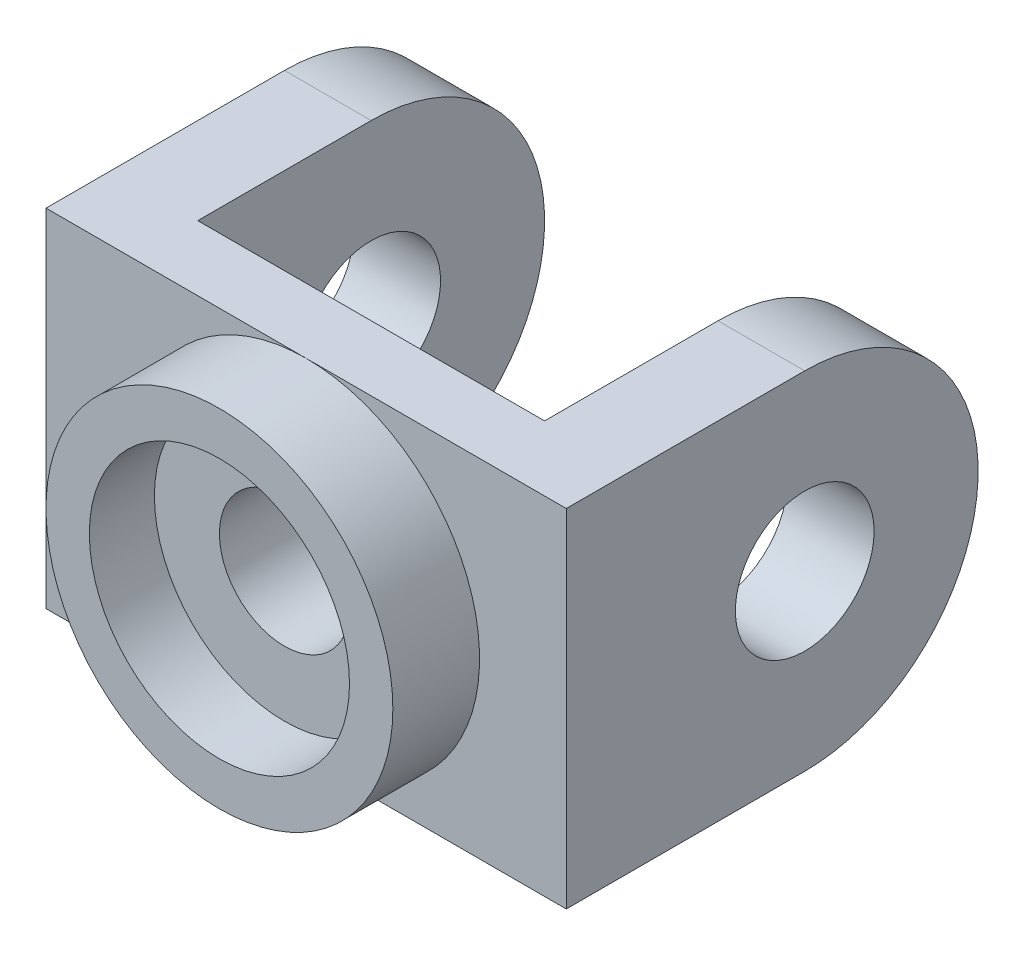
ISO-10303-21;
HEADER;
FILE_DESCRIPTION(('STEP AP214'),'2;1');
FILE_NAME('part.step','',(''),(''),'','','');
FILE_SCHEMA(('AUTOMOTIVE_DESIGN { 1 0 10303 214 1 1 1 1 }'));
ENDSEC;
DATA;
#1=APPLICATION_CONTEXT('core data for automotive mechanical design processes');
#2=APPLICATION_PROTOCOL_DEFINITION('international standard','automotive_design',2000,#1);
#3=PRODUCT_CONTEXT('',#1,'mechanical');
#4=PRODUCT('Part','Part','',(#3));
#5=PRODUCT_RELATED_PRODUCT_CATEGORY('part','',(#4));
#6=PRODUCT_DEFINITION_FORMATION('','',#4);
#7=PRODUCT_DEFINITION_CONTEXT('part definition',#1,'design');
#8=PRODUCT_DEFINITION('design','',#6,#7);
#9=PRODUCT_DEFINITION_SHAPE('','',#8);
#10=(LENGTH_UNIT() NAMED_UNIT(*) SI_UNIT(.MILLI.,.METRE.));
#11=(NAMED_UNIT(*) PLANE_ANGLE_UNIT() SI_UNIT($,.RADIAN.));
#12=(NAMED_UNIT(*) SI_UNIT($,.STERADIAN.) SOLID_ANGLE_UNIT());
#13=UNCERTAINTY_MEASURE_WITH_UNIT(LENGTH_MEASURE(1.E-05),#10,'distance_accuracy_value','');
#14=(GEOMETRIC_REPRESENTATION_CONTEXT(3) GLOBAL_UNCERTAINTY_ASSIGNED_CONTEXT((#13)) GLOBAL_UNIT_ASSIGNED_CONTEXT((#10,
#11,#12)) REPRESENTATION_CONTEXT('',''));
#15=CARTESIAN_POINT('',(0.,0.,0.));
#16=DIRECTION('',(0.,0.,1.));
#17=DIRECTION('',(1.,0.,0.));
#18=AXIS2_PLACEMENT_3D('',#15,#16,#17);
#19=CARTESIAN_POINT('',(0.,0.,0.));
#20=DIRECTION('',(0.,0.,-1.));
#21=DIRECTION('',(-1.,0.,0.));
#22=AXIS2_PLACEMENT_3D('',#19,#20,#21);
#23=PLANE('',#22);
#24=CARTESIAN_POINT('',(0.,0.,0.));
#25=DIRECTION('',(0.,0.,-1.));
#26=DIRECTION('',(-1.,0.,0.));
#27=AXIS2_PLACEMENT_3D('',#24,#25,#26);
#28=CIRCLE('',#27,15.);
#29=CARTESIAN_POINT('',(-15.,0.,0.));
#30=VERTEX_POINT('',#29);
#31=EDGE_CURVE('E185',#30,#30,#28,.T.);
#32=ORIENTED_EDGE('',*,*,#31,.F.);
#33=EDGE_LOOP('',(#32));
#34=FACE_BOUND('',#33,.T.);
#35=DIRECTION('',(1.,0.,0.));
#36=VECTOR('',#35,1.);
#37=CARTESIAN_POINT('',(-60.,-40.,0.));
#38=LINE('',#37,#36);
#39=CARTESIAN_POINT('',(-40.,-40.,0.));
#40=VERTEX_POINT('',#39);
#41=CARTESIAN_POINT('',(40.,-40.,0.));
#42=VERTEX_POINT('',#41);
#43=EDGE_CURVE('E53',#40,#42,#38,.T.);
#44=ORIENTED_EDGE('',*,*,#43,.F.);
#45=DIRECTION('',(0.,1.,0.));
#46=VECTOR('',#45,1.);
#47=CARTESIAN_POINT('',(-40.,0.,0.));
#48=LINE('',#47,#46);
#49=CARTESIAN_POINT('',(-40.,40.,0.));
#50=VERTEX_POINT('',#49);
#51=EDGE_CURVE('E132',#40,#50,#48,.T.);
#52=ORIENTED_EDGE('',*,*,#51,.T.);
#53=DIRECTION('',(-1.,0.,0.));
#54=VECTOR('',#53,1.);
#55=CARTESIAN_POINT('',(-60.,40.,0.));
#56=LINE('',#55,#54);
#57=CARTESIAN_POINT('',(40.,40.,0.));
#58=VERTEX_POINT('',#57);
#59=EDGE_CURVE('E187',#58,#50,#56,.T.);
#60=ORIENTED_EDGE('',*,*,#59,.F.);
#61=DIRECTION('',(0.,-1.,0.));
#62=VECTOR('',#61,1.);
#63=CARTESIAN_POINT('',(40.,-40.,0.));
#64=LINE('',#63,#62);
#65=EDGE_CURVE('E152',#58,#42,#64,.T.);
#66=ORIENTED_EDGE('',*,*,#65,.T.);
#67=EDGE_LOOP('',(#44,#52,#60,#66));
#68=FACE_BOUND('',#67,.T.);
#69=ADVANCED_FACE('F39',(#34,#68),#23,.T.);
#70=CARTESIAN_POINT('',(0.,0.,15.));
#71=DIRECTION('',(0.,0.,-1.));
#72=DIRECTION('',(-1.,0.,0.));
#73=AXIS2_PLACEMENT_3D('',#70,#71,#72);
#74=PLANE('',#73);
#75=DIRECTION('',(1.,0.,0.));
#76=VECTOR('',#75,1.);
#77=CARTESIAN_POINT('',(-60.,-40.,15.));
#78=LINE('',#77,#76);
#79=CARTESIAN_POINT('',(-60.,-40.,15.));
#80=VERTEX_POINT('',#79);
#81=CARTESIAN_POINT('',(0.,-40.,15.));
#82=VERTEX_POINT('',#81);
#83=EDGE_CURVE('E198',#80,#82,#78,.T.);
#84=ORIENTED_EDGE('',*,*,#83,.T.);
#85=CARTESIAN_POINT('',(0.,0.,15.));
#86=DIRECTION('',(0.,0.,1.));
#87=DIRECTION('',(1.,0.,0.));
#88=AXIS2_PLACEMENT_3D('',#85,#86,#87);
#89=CIRCLE('',#88,40.);
#90=CARTESIAN_POINT('',(0.,40.,15.));
#91=VERTEX_POINT('',#90);
#92=EDGE_CURVE('E62',#91,#82,#89,.T.);
#93=ORIENTED_EDGE('',*,*,#92,.F.);
#94=DIRECTION('',(-1.,0.,0.));
#95=VECTOR('',#94,1.);
#96=CARTESIAN_POINT('',(-60.,40.,15.));
#97=LINE('',#96,#95);
#98=CARTESIAN_POINT('',(-60.,40.,15.));
#99=VERTEX_POINT('',#98);
#100=EDGE_CURVE('E188',#91,#99,#97,.T.);
#101=ORIENTED_EDGE('',*,*,#100,.T.);
#102=DIRECTION('',(0.,-1.,0.));
#103=VECTOR('',#102,1.);
#104=CARTESIAN_POINT('',(-60.,-40.,15.));
#105=LINE('',#104,#103);
#106=EDGE_CURVE('E194',#99,#80,#105,.T.);
#107=ORIENTED_EDGE('',*,*,#106,.T.);
#108=EDGE_LOOP('',(#84,#93,#101,#107));
#109=FACE_BOUND('',#108,.T.);
#110=ADVANCED_FACE('F244',(#109),#74,.F.);
#111=CARTESIAN_POINT('',(60.,-40.,15.));
#112=DIRECTION('',(-1.,0.,0.));
#113=DIRECTION('',(0.,0.,1.));
#114=AXIS2_PLACEMENT_3D('',#111,#112,#113);
#115=PLANE('',#114);
#116=DIRECTION('',(0.,0.,-1.));
#117=VECTOR('',#116,1.);
#118=CARTESIAN_POINT('',(60.,-40.,15.));
#119=LINE('',#118,#117);
#120=CARTESIAN_POINT('',(60.,-40.,15.));
#121=VERTEX_POINT('',#120);
#122=CARTESIAN_POINT('',(60.,-40.,-40.));
#123=VERTEX_POINT('',#122);
#124=EDGE_CURVE('E196',#121,#123,#119,.T.);
#125=ORIENTED_EDGE('',*,*,#124,.T.);
#126=CARTESIAN_POINT('',(60.,0.,-40.));
#127=DIRECTION('',(1.,0.,0.));
#128=DIRECTION('',(0.,0.,-1.));
#129=AXIS2_PLACEMENT_3D('',#126,#127,#128);
#130=CIRCLE('',#129,40.);
#131=CARTESIAN_POINT('',(60.,40.,-40.));
#132=VERTEX_POINT('',#131);
#133=EDGE_CURVE('E151',#123,#132,#130,.T.);
#134=ORIENTED_EDGE('',*,*,#133,.T.);
#135=DIRECTION('',(0.,0.,-1.));
#136=VECTOR('',#135,1.);
#137=CARTESIAN_POINT('',(60.,40.,15.));
#138=LINE('',#137,#136);
#139=CARTESIAN_POINT('',(60.,40.,15.));
#140=VERTEX_POINT('',#139);
#141=EDGE_CURVE('E202',#140,#132,#138,.T.);
#142=ORIENTED_EDGE('',*,*,#141,.F.);
#143=DIRECTION('',(0.,1.,0.));
#144=VECTOR('',#143,1.);
#145=CARTESIAN_POINT('',(60.,-40.,15.));
#146=LINE('',#145,#144);
#147=EDGE_CURVE('E189',#121,#140,#146,.T.);
#148=ORIENTED_EDGE('',*,*,#147,.F.);
#149=EDGE_LOOP('',(#125,#134,#142,#148));
#150=FACE_BOUND('',#149,.T.);
#151=CARTESIAN_POINT('',(60.,0.,-40.));
#152=DIRECTION('',(1.,0.,0.));
#153=DIRECTION('',(0.,0.,-1.));
#154=AXIS2_PLACEMENT_3D('',#151,#152,#153);
#155=CIRCLE('',#154,16.);
#156=CARTESIAN_POINT('',(60.,0.,-56.));
#157=VERTEX_POINT('',#156);
#158=EDGE_CURVE('E150',#157,#157,#155,.T.);
#159=ORIENTED_EDGE('',*,*,#158,.F.);
#160=EDGE_LOOP('',(#159));
#161=FACE_BOUND('',#160,.T.);
#162=ADVANCED_FACE('F41',(#150,#161),#115,.F.);
#163=CARTESIAN_POINT('',(-60.,40.,15.));
#164=DIRECTION('',(0.,-1.,0.));
#165=DIRECTION('',(0.,0.,-1.));
#166=AXIS2_PLACEMENT_3D('',#163,#164,#165);
#167=PLANE('',#166);
#168=DIRECTION('',(0.,0.,-1.));
#169=VECTOR('',#168,1.);
#170=CARTESIAN_POINT('',(-60.,40.,15.));
#171=LINE('',#170,#169);
#172=CARTESIAN_POINT('',(-60.,40.,-40.));
#173=VERTEX_POINT('',#172);
#174=EDGE_CURVE('E204',#99,#173,#171,.T.);
#175=ORIENTED_EDGE('',*,*,#174,.F.);
#176=ORIENTED_EDGE('',*,*,#100,.F.);
#177=EDGE_CURVE('E191',#140,#91,#97,.T.);
#178=ORIENTED_EDGE('',*,*,#177,.F.);
#179=ORIENTED_EDGE('',*,*,#141,.T.);
#180=DIRECTION('',(1.,0.,0.));
#181=VECTOR('',#180,1.);
#182=CARTESIAN_POINT('',(40.,40.,-40.));
#183=LINE('',#182,#181);
#184=CARTESIAN_POINT('',(40.,40.,-40.));
#185=VERTEX_POINT('',#184);
#186=EDGE_CURVE('E169',#185,#132,#183,.T.);
#187=ORIENTED_EDGE('',*,*,#186,.F.);
#188=DIRECTION('',(0.,0.,1.));
#189=VECTOR('',#188,1.);
#190=CARTESIAN_POINT('',(40.,40.,0.));
#191=LINE('',#190,#189);
#192=EDGE_CURVE('E165',#185,#58,#191,.T.);
#193=ORIENTED_EDGE('',*,*,#192,.T.);
#194=ORIENTED_EDGE('',*,*,#59,.T.);
#195=DIRECTION('',(0.,0.,-1.));
#196=VECTOR('',#195,1.);
#197=CARTESIAN_POINT('',(-40.,40.,-40.));
#198=LINE('',#197,#196);
#199=CARTESIAN_POINT('',(-40.,40.,-40.));
#200=VERTEX_POINT('',#199);
#201=EDGE_CURVE('E124',#50,#200,#198,.T.);
#202=ORIENTED_EDGE('',*,*,#201,.T.);
#203=DIRECTION('',(-1.,0.,0.));
#204=VECTOR('',#203,1.);
#205=CARTESIAN_POINT('',(-40.,40.,-40.));
#206=LINE('',#205,#204);
#207=EDGE_CURVE('E122',#200,#173,#206,.T.);
#208=ORIENTED_EDGE('',*,*,#207,.T.);
#209=EDGE_LOOP('',(#175,#176,#178,#179,#187,#193,#194,#202,#208));
#210=FACE_BOUND('',#209,.T.);
#211=ADVANCED_FACE('F221',(#210),#167,.F.);
#212=CARTESIAN_POINT('',(-60.,-40.,15.));
#213=DIRECTION('',(1.,0.,0.));
#214=DIRECTION('',(0.,0.,-1.));
#215=AXIS2_PLACEMENT_3D('',#212,#213,#214);
#216=PLANE('',#215);
#217=ORIENTED_EDGE('',*,*,#174,.T.);
#218=CARTESIAN_POINT('',(-60.,0.,-40.));
#219=DIRECTION('',(-1.,0.,0.));
#220=DIRECTION('',(0.,0.,1.));
#221=AXIS2_PLACEMENT_3D('',#218,#219,#220);
#222=CIRCLE('',#221,40.);
#223=CARTESIAN_POINT('',(-60.,-40.,-40.));
#224=VERTEX_POINT('',#223);
#225=EDGE_CURVE('E136',#173,#224,#222,.T.);
#226=ORIENTED_EDGE('',*,*,#225,.T.);
#227=DIRECTION('',(0.,0.,-1.));
#228=VECTOR('',#227,1.);
#229=CARTESIAN_POINT('',(-60.,-40.,15.));
#230=LINE('',#229,#228);
#231=EDGE_CURVE('E119',#80,#224,#230,.T.);
#232=ORIENTED_EDGE('',*,*,#231,.F.);
#233=ORIENTED_EDGE('',*,*,#106,.F.);
#234=EDGE_LOOP('',(#217,#226,#232,#233));
#235=FACE_BOUND('',#234,.T.);
#236=CARTESIAN_POINT('',(-60.,0.,-40.));
#237=DIRECTION('',(-1.,0.,0.));
#238=DIRECTION('',(0.,0.,1.));
#239=AXIS2_PLACEMENT_3D('',#236,#237,#238);
#240=CIRCLE('',#239,16.);
#241=CARTESIAN_POINT('',(-60.,0.,-24.));
#242=VERTEX_POINT('',#241);
#243=EDGE_CURVE('E143',#242,#242,#240,.T.);
#244=ORIENTED_EDGE('',*,*,#243,.F.);
#245=EDGE_LOOP('',(#244));
#246=FACE_BOUND('',#245,.T.);
#247=ADVANCED_FACE('F254',(#235,#246),#216,.F.);
#248=CARTESIAN_POINT('',(-60.,-40.,15.));
#249=DIRECTION('',(0.,1.,0.));
#250=DIRECTION('',(0.,0.,1.));
#251=AXIS2_PLACEMENT_3D('',#248,#249,#250);
#252=PLANE('',#251);
#253=ORIENTED_EDGE('',*,*,#231,.T.);
#254=DIRECTION('',(-1.,0.,0.));
#255=VECTOR('',#254,1.);
#256=CARTESIAN_POINT('',(-40.,-40.,-40.));
#257=LINE('',#256,#255);
#258=CARTESIAN_POINT('',(-40.,-40.,-40.));
#259=VERTEX_POINT('',#258);
#260=EDGE_CURVE('E112',#259,#224,#257,.T.);
#261=ORIENTED_EDGE('',*,*,#260,.F.);
#262=DIRECTION('',(0.,0.,1.));
#263=VECTOR('',#262,1.);
#264=CARTESIAN_POINT('',(-40.,-40.,-40.));
#265=LINE('',#264,#263);
#266=EDGE_CURVE('E111',#259,#40,#265,.T.);
#267=ORIENTED_EDGE('',*,*,#266,.T.);
#268=ORIENTED_EDGE('',*,*,#43,.T.);
#269=DIRECTION('',(0.,0.,-1.));
#270=VECTOR('',#269,1.);
#271=CARTESIAN_POINT('',(40.,-40.,0.));
#272=LINE('',#271,#270);
#273=CARTESIAN_POINT('',(40.,-40.,-40.));
#274=VERTEX_POINT('',#273);
#275=EDGE_CURVE('E160',#42,#274,#272,.T.);
#276=ORIENTED_EDGE('',*,*,#275,.T.);
#277=DIRECTION('',(1.,0.,0.));
#278=VECTOR('',#277,1.);
#279=CARTESIAN_POINT('',(40.,-40.,-40.));
#280=LINE('',#279,#278);
#281=EDGE_CURVE('E164',#274,#123,#280,.T.);
#282=ORIENTED_EDGE('',*,*,#281,.T.);
#283=ORIENTED_EDGE('',*,*,#124,.F.);
#284=EDGE_CURVE('E195',#82,#121,#78,.T.);
#285=ORIENTED_EDGE('',*,*,#284,.F.);
#286=ORIENTED_EDGE('',*,*,#83,.F.);
#287=EDGE_LOOP('',(#253,#261,#267,#268,#276,#282,#283,#285,#286));
#288=FACE_BOUND('',#287,.T.);
#289=ADVANCED_FACE('F114',(#288),#252,.F.);
#290=EDGE_CURVE('E50',#82,#91,#89,.T.);
#291=ORIENTED_EDGE('',*,*,#290,.F.);
#292=ORIENTED_EDGE('',*,*,#284,.T.);
#293=ORIENTED_EDGE('',*,*,#147,.T.);
#294=ORIENTED_EDGE('',*,*,#177,.T.);
#295=EDGE_LOOP('',(#291,#292,#293,#294));
#296=FACE_BOUND('',#295,.T.);
#297=ADVANCED_FACE('F215',(#296),#74,.F.);
#298=CARTESIAN_POINT('',(0.,0.,15.));
#299=DIRECTION('',(0.,0.,-1.));
#300=DIRECTION('',(-1.,0.,0.));
#301=AXIS2_PLACEMENT_3D('',#298,#299,#300);
#302=CYLINDRICAL_SURFACE('',#301,15.);
#303=ORIENTED_EDGE('',*,*,#31,.T.);
#304=EDGE_LOOP('',(#303));
#305=FACE_BOUND('',#304,.T.);
#306=CARTESIAN_POINT('',(0.,0.,20.));
#307=DIRECTION('',(0.,0.,1.));
#308=DIRECTION('',(1.,0.,0.));
#309=AXIS2_PLACEMENT_3D('',#306,#307,#308);
#310=CIRCLE('',#309,15.);
#311=CARTESIAN_POINT('',(15.,0.,20.));
#312=VERTEX_POINT('',#311);
#313=EDGE_CURVE('E172',#312,#312,#310,.T.);
#314=ORIENTED_EDGE('',*,*,#313,.T.);
#315=EDGE_LOOP('',(#314));
#316=FACE_BOUND('',#315,.T.);
#317=ADVANCED_FACE('F373',(#305,#316),#302,.F.);
#318=CARTESIAN_POINT('',(0.,0.,35.));
#319=DIRECTION('',(0.,0.,1.));
#320=DIRECTION('',(1.,0.,0.));
#321=AXIS2_PLACEMENT_3D('',#318,#319,#320);
#322=PLANE('',#321);
#323=CARTESIAN_POINT('',(0.,0.,35.));
#324=DIRECTION('',(0.,0.,1.));
#325=DIRECTION('',(1.,0.,0.));
#326=AXIS2_PLACEMENT_3D('',#323,#324,#325);
#327=CIRCLE('',#326,40.);
#328=CARTESIAN_POINT('',(40.,0.,35.));
#329=VERTEX_POINT('',#328);
#330=EDGE_CURVE('E178',#329,#329,#327,.T.);
#331=ORIENTED_EDGE('',*,*,#330,.T.);
#332=EDGE_LOOP('',(#331));
#333=FACE_BOUND('',#332,.T.);
#334=CARTESIAN_POINT('',(0.,0.,35.));
#335=DIRECTION('',(0.,0.,1.));
#336=DIRECTION('',(1.,0.,0.));
#337=AXIS2_PLACEMENT_3D('',#334,#335,#336);
#338=CIRCLE('',#337,30.);
#339=CARTESIAN_POINT('',(30.,0.,35.));
#340=VERTEX_POINT('',#339);
#341=EDGE_CURVE('E176',#340,#340,#338,.T.);
#342=ORIENTED_EDGE('',*,*,#341,.F.);
#343=EDGE_LOOP('',(#342));
#344=FACE_BOUND('',#343,.T.);
#345=ADVANCED_FACE('F348',(#333,#344),#322,.T.);
#346=CARTESIAN_POINT('',(0.,0.,35.));
#347=DIRECTION('',(0.,0.,-1.));
#348=DIRECTION('',(-1.,0.,0.));
#349=AXIS2_PLACEMENT_3D('',#346,#347,#348);
#350=CYLINDRICAL_SURFACE('',#349,40.);
#351=ORIENTED_EDGE('',*,*,#330,.F.);
#352=EDGE_LOOP('',(#351));
#353=FACE_BOUND('',#352,.T.);
#354=ORIENTED_EDGE('',*,*,#92,.T.);
#355=ORIENTED_EDGE('',*,*,#290,.T.);
#356=EDGE_LOOP('',(#354,#355));
#357=FACE_BOUND('',#356,.T.);
#358=ADVANCED_FACE('F207',(#353,#357),#350,.T.);
#359=CARTESIAN_POINT('',(0.,0.,35.));
#360=DIRECTION('',(0.,0.,-1.));
#361=DIRECTION('',(-1.,0.,0.));
#362=AXIS2_PLACEMENT_3D('',#359,#360,#361);
#363=CYLINDRICAL_SURFACE('',#362,30.);
#364=CARTESIAN_POINT('',(0.,0.,20.));
#365=DIRECTION('',(0.,0.,1.));
#366=DIRECTION('',(1.,0.,0.));
#367=AXIS2_PLACEMENT_3D('',#364,#365,#366);
#368=CIRCLE('',#367,30.);
#369=CARTESIAN_POINT('',(30.,0.,20.));
#370=VERTEX_POINT('',#369);
#371=EDGE_CURVE('E11',#370,#370,#368,.T.);
#372=ORIENTED_EDGE('',*,*,#371,.F.);
#373=EDGE_LOOP('',(#372));
#374=FACE_BOUND('',#373,.T.);
#375=ORIENTED_EDGE('',*,*,#341,.T.);
#376=EDGE_LOOP('',(#375));
#377=FACE_BOUND('',#376,.T.);
#378=ADVANCED_FACE('F349',(#374,#377),#363,.F.);
#379=CARTESIAN_POINT('',(0.,0.,20.));
#380=DIRECTION('',(0.,0.,1.));
#381=DIRECTION('',(1.,0.,0.));
#382=AXIS2_PLACEMENT_3D('',#379,#380,#381);
#383=PLANE('',#382);
#384=ORIENTED_EDGE('',*,*,#371,.T.);
#385=EDGE_LOOP('',(#384));
#386=FACE_BOUND('',#385,.T.);
#387=ORIENTED_EDGE('',*,*,#313,.F.);
#388=EDGE_LOOP('',(#387));
#389=FACE_BOUND('',#388,.T.);
#390=ADVANCED_FACE('F239',(#386,#389),#383,.T.);
#391=CARTESIAN_POINT('',(40.,0.,-40.));
#392=DIRECTION('',(1.,0.,0.));
#393=DIRECTION('',(0.,0.,-1.));
#394=AXIS2_PLACEMENT_3D('',#391,#392,#393);
#395=CYLINDRICAL_SURFACE('',#394,40.);
#396=ORIENTED_EDGE('',*,*,#133,.F.);
#397=ORIENTED_EDGE('',*,*,#281,.F.);
#398=CARTESIAN_POINT('',(40.,0.,-40.));
#399=DIRECTION('',(1.,0.,0.));
#400=DIRECTION('',(0.,0.,-1.));
#401=AXIS2_PLACEMENT_3D('',#398,#399,#400);
#402=CIRCLE('',#401,40.);
#403=EDGE_CURVE('E157',#274,#185,#402,.T.);
#404=ORIENTED_EDGE('',*,*,#403,.T.);
#405=ORIENTED_EDGE('',*,*,#186,.T.);
#406=EDGE_LOOP('',(#396,#397,#404,#405));
#407=FACE_BOUND('',#406,.T.);
#408=ADVANCED_FACE('F219',(#407),#395,.T.);
#409=CARTESIAN_POINT('',(40.,0.,-40.));
#410=DIRECTION('',(1.,0.,0.));
#411=DIRECTION('',(0.,0.,-1.));
#412=AXIS2_PLACEMENT_3D('',#409,#410,#411);
#413=PLANE('',#412);
#414=CARTESIAN_POINT('',(40.,0.,-40.));
#415=DIRECTION('',(1.,0.,0.));
#416=DIRECTION('',(0.,0.,-1.));
#417=AXIS2_PLACEMENT_3D('',#414,#415,#416);
#418=CIRCLE('',#417,16.);
#419=CARTESIAN_POINT('',(40.,0.,-56.));
#420=VERTEX_POINT('',#419);
#421=EDGE_CURVE('E146',#420,#420,#418,.T.);
#422=ORIENTED_EDGE('',*,*,#421,.T.);
#423=EDGE_LOOP('',(#422));
#424=FACE_BOUND('',#423,.T.);
#425=ORIENTED_EDGE('',*,*,#65,.F.);
#426=ORIENTED_EDGE('',*,*,#192,.F.);
#427=ORIENTED_EDGE('',*,*,#403,.F.);
#428=ORIENTED_EDGE('',*,*,#275,.F.);
#429=EDGE_LOOP('',(#425,#426,#427,#428));
#430=FACE_BOUND('',#429,.T.);
#431=ADVANCED_FACE('F230',(#424,#430),#413,.F.);
#432=CARTESIAN_POINT('',(40.,0.,-40.));
#433=DIRECTION('',(1.,0.,0.));
#434=DIRECTION('',(0.,0.,-1.));
#435=AXIS2_PLACEMENT_3D('',#432,#433,#434);
#436=CYLINDRICAL_SURFACE('',#435,16.);
#437=ORIENTED_EDGE('',*,*,#421,.F.);
#438=EDGE_LOOP('',(#437));
#439=FACE_BOUND('',#438,.T.);
#440=ORIENTED_EDGE('',*,*,#158,.T.);
#441=EDGE_LOOP('',(#440));
#442=FACE_BOUND('',#441,.T.);
#443=ADVANCED_FACE('F228',(#439,#442),#436,.F.);
#444=CARTESIAN_POINT('',(-40.,0.,-40.));
#445=DIRECTION('',(-1.,0.,0.));
#446=DIRECTION('',(0.,0.,1.));
#447=AXIS2_PLACEMENT_3D('',#444,#445,#446);
#448=CYLINDRICAL_SURFACE('',#447,40.);
#449=ORIENTED_EDGE('',*,*,#225,.F.);
#450=ORIENTED_EDGE('',*,*,#207,.F.);
#451=CARTESIAN_POINT('',(-40.,0.,-40.));
#452=DIRECTION('',(-1.,0.,0.));
#453=DIRECTION('',(0.,0.,1.));
#454=AXIS2_PLACEMENT_3D('',#451,#452,#453);
#455=CIRCLE('',#454,40.);
#456=EDGE_CURVE('E129',#200,#259,#455,.T.);
#457=ORIENTED_EDGE('',*,*,#456,.T.);
#458=ORIENTED_EDGE('',*,*,#260,.T.);
#459=EDGE_LOOP('',(#449,#450,#457,#458));
#460=FACE_BOUND('',#459,.T.);
#461=ADVANCED_FACE('F131',(#460),#448,.T.);
#462=CARTESIAN_POINT('',(-40.,0.,-40.));
#463=DIRECTION('',(-1.,0.,0.));
#464=DIRECTION('',(0.,0.,1.));
#465=AXIS2_PLACEMENT_3D('',#462,#463,#464);
#466=PLANE('',#465);
#467=ORIENTED_EDGE('',*,*,#51,.F.);
#468=ORIENTED_EDGE('',*,*,#266,.F.);
#469=ORIENTED_EDGE('',*,*,#456,.F.);
#470=ORIENTED_EDGE('',*,*,#201,.F.);
#471=EDGE_LOOP('',(#467,#468,#469,#470));
#472=FACE_BOUND('',#471,.T.);
#473=CARTESIAN_POINT('',(-40.,0.,-40.));
#474=DIRECTION('',(-1.,0.,0.));
#475=DIRECTION('',(0.,0.,1.));
#476=AXIS2_PLACEMENT_3D('',#473,#474,#475);
#477=CIRCLE('',#476,16.);
#478=CARTESIAN_POINT('',(-40.,0.,-24.));
#479=VERTEX_POINT('',#478);
#480=EDGE_CURVE('E139',#479,#479,#477,.T.);
#481=ORIENTED_EDGE('',*,*,#480,.T.);
#482=EDGE_LOOP('',(#481));
#483=FACE_BOUND('',#482,.T.);
#484=ADVANCED_FACE('F130',(#472,#483),#466,.F.);
#485=CARTESIAN_POINT('',(-40.,0.,-40.));
#486=DIRECTION('',(-1.,0.,0.));
#487=DIRECTION('',(0.,0.,1.));
#488=AXIS2_PLACEMENT_3D('',#485,#486,#487);
#489=CYLINDRICAL_SURFACE('',#488,16.);
#490=ORIENTED_EDGE('',*,*,#480,.F.);
#491=EDGE_LOOP('',(#490));
#492=FACE_BOUND('',#491,.T.);
#493=ORIENTED_EDGE('',*,*,#243,.T.);
#494=EDGE_LOOP('',(#493));
#495=FACE_BOUND('',#494,.T.);
#496=ADVANCED_FACE('F328',(#492,#495),#489,.F.);
#497=CLOSED_SHELL('',(#69,#110,#162,#211,#247,#289,#297,#317,#345,#358,#378,#390,#408,#431,#443,
#461,#484,#496));
#498=MANIFOLD_SOLID_BREP('B2',#497);
#499=ADVANCED_BREP_SHAPE_REPRESENTATION('',(#18,#498),#14);
#500=SHAPE_DEFINITION_REPRESENTATION(#9,#499);
ENDSEC;
END-ISO-10303-21;
